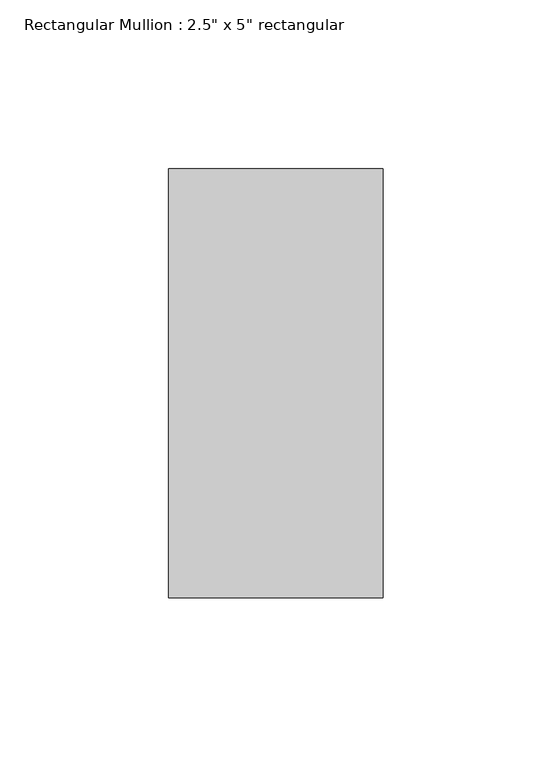
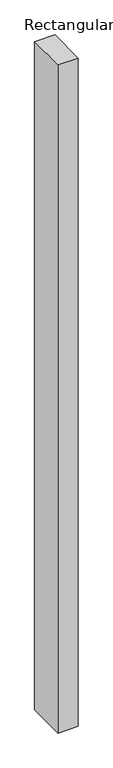
"""IFC4 building model written with IfcOpenShell, lengths in millimetres: member geometry."""

from ifc_helpers import new_model, si_unit, frame, origin, place, context, project, spatial, polyline, outline, extrude, source, transform, mapped, element, save


def member_5c0bf374(model_context):
    return source(origin(), model_context, "Body", "SweptSolid", [
        extrude(outline(polyline([(0.0, 63.5), (0.0, -63.5), (-63.5, -63.5), (-63.5, 63.5), (0.0, 63.5)])), frame((0.0, 0.0, -2222.5), z_axis=(0.0, 0.0, 1.0), x_axis=(1.0, 0.0, 0.0)), (0.0, 0.0, 1.0), 2222.5),
    ])


if __name__ == "__main__":
    model = new_model("IFC4")
    model_context = context("Model", 3, world=origin())
    ifc_project = project(units=[si_unit("LENGTHUNIT", "METRE", prefix="MILLI")], contexts=[model_context])
    site = spatial("IfcSite", under=ifc_project)
    building = spatial("IfcBuilding", under=site)
    placement = place(None, origin())
    member_shape = member_5c0bf374(model_context)
    element("IfcMember", 1, ObjectType="Rectangular Mullion : 2.5\" x 5\" rectangular", at=placement, inside=building, context=model_context, shape_type="MappedRepresentation", body=[
        mapped(member_shape, transform((0.0, 0.0, 0.0), x_axis=(1.0, 0.0, 0.0), y_axis=(0.0, 1.0, 0.0), z_axis=(0.0, 0.0, 1.0))),
    ])
    save(model, "model.ifc")

# Revit data of these elements
# Type "Rectangular Mullion : 2.5\" x 5\" rectangular"
#   built-in parameter 1007304 = 0.416667 (stored number, unit not read)
#   built-in parameter 1007301 = 0.104167 (stored number, unit not read)
#   built-in parameter 1007300 = 0.104167 (stored number, unit not read)
# Element 1 (IfcMember, "Rectangular Mullion : 2.5\" x 5\" rectangular")
#   Materials on its faces: "Aluminum"
# Materials
#   "Aluminum": class "Metal", colour RGB 247 247 247, transparency 0, Description = "Aluminum 6061", Cost = 0
